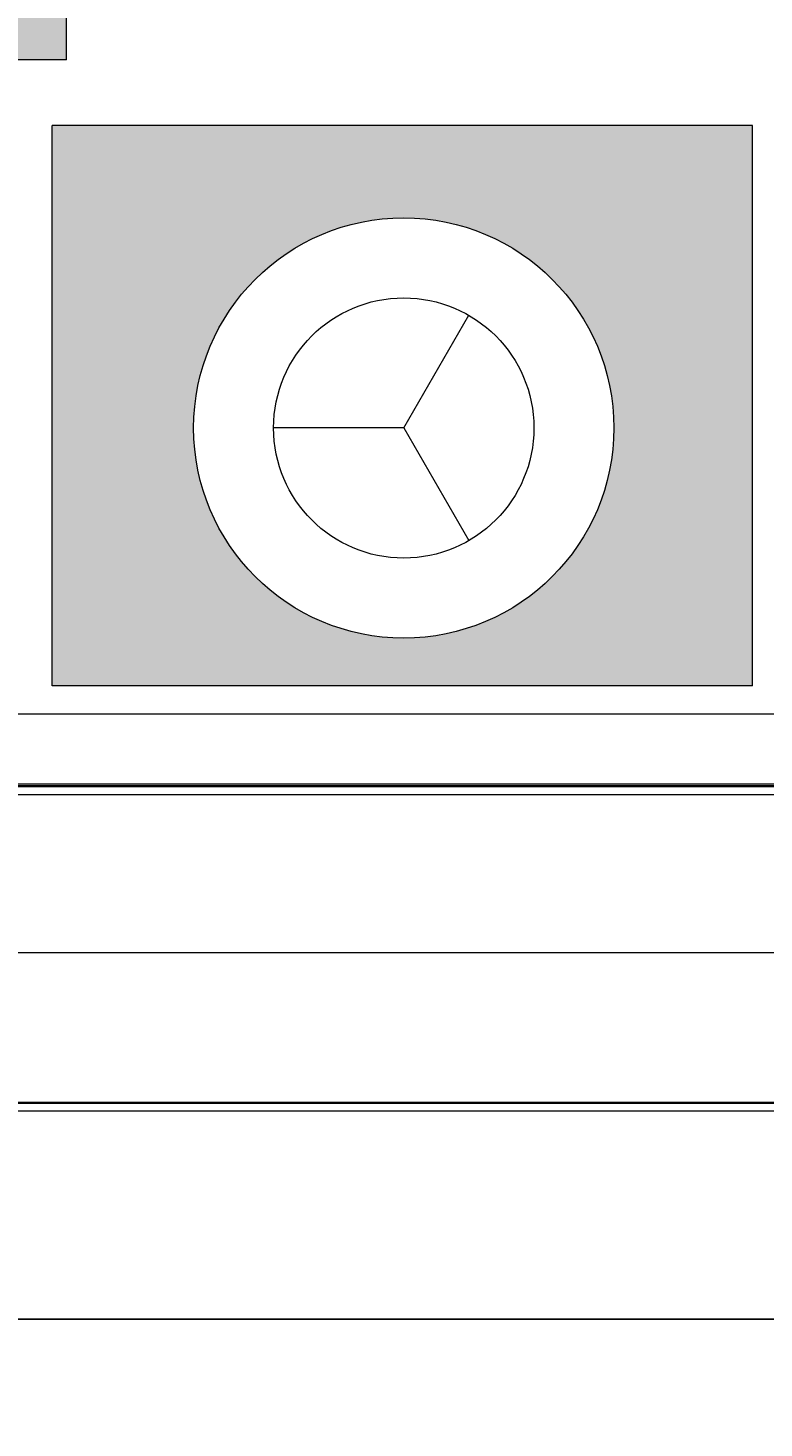
# Model space of a CAD drawing. Units: millimetres. Extents: x 27017497 to 27018854, y 7058029 to 7059154.
# Tile 25 of 91: x 27017732 to 27017753, y 7058124 to 7058163. Entities that reach past the tile are written whole.
import ezdxf

# ---------------------------------------------------------------- set-up
doc = ezdxf.new("R2010")
doc.units = ezdxf.units.MM
for name, color, linetype, lineweight in [('A-ANNO-DIMS', 2, 'Continuous', 18), ('A-FURN', 8, 'Continuous', 18), ('A-GLAZ', 4, 'Continuous', 18), ('A-WALL', 7, 'Continuous', 35)]:
    doc.layers.add(name, color=color, linetype=linetype, lineweight=lineweight)
doc.layers.add('A-FURN-PATT', color=177, linetype='Continuous', lineweight=13, true_color=0x293189)
doc.styles.get("Standard").update_dxf_attribs({"font": 'arial.ttf'})
doc.dimstyles.get("Standard").update_dxf_attribs({"dimtxt": 0.18, "dimasz": 0.18, "dimexe": 0.18, "dimexo": 0.0625, "dimgap": 0.09, "dimtad": 0, "dimtih": 1, "dimtoh": 1, "dimdec": 4, "dimzin": 0, "dimdsep": 46, "dimtxsty": 'Standard', "dimcen": 0.09, "dimadec": 0, "dimazin": 0, "dimtfac": 1, "dimtdec": 4, "dimtofl": 0, "dimtmove": 0, "dimatfit": 3, "dimfxl": 1, "dimtolj": 1, "dimtzin": 0, "dimarcsym": 0})

# ---------------------------------------------------------------- blocks, each defined once
blk = doc.blocks.new('CAMMAT')
for p, q in [((1.27313, 0), (-1.27313, 0)), ((1.27313, -0.05), (-1.27313, -0.05)), ((-1.18, -0.07), (-1.18, -0.47)), ((-1.18, -0.07), (-0.68, -0.07)), ((-0.68, -0.07), (-0.68, -0.47)), ((-0.93104, -0.2541), (-0.97748, -0.17366)), ((-0.93104, -0.2541), (-0.97748, -0.33455)), ((-0.93104, -0.2541), (-0.83815, -0.2541)), ((-1.18, -0.47), (-0.68, -0.47)), ((-0.6904, -0.51693), (-0.6904, -0.8)), ((-0.6904, -0.51693), (0.68256, -0.51693))]:
    blk.add_line(p, q)
for radius in [0.15, 0.09289]:
    blk.add_circle((-0.93104, -0.2541), radius)
blk = doc.blocks.new('WINDOW-SINGLE-LIGHT')
blk.add_lwpolyline([(36, 4.5), (36, 0), (0, 0), (0, 9), (36, 9), (36, 4.5), (0, 4.5)])
blk = doc.blocks.new('*D25')
at = {"layer": 'A-ANNO-DIMS', "color": 0, "lineweight": -2, "transparency": 16777216}
for p, q in [((27017654.932, 7058141.917), (27017654.932, 7058126.587)), ((27017756.349, 7058141.917), (27017756.349, 7058126.587)), ((27017655.112, 7058126.767), (27017704.753, 7058126.767)), ((27017756.169, 7058126.767), (27017706.528, 7058126.767))]:
    blk.add_line(p, q, dxfattribs=at)
at = {"layer": 'A-ANNO-DIMS', "color": 0, "transparency": 16777216}
for points in [[(27017655.112, 7058126.797), (27017655.112, 7058126.737), (27017654.932, 7058126.767)], [(27017756.169, 7058126.797), (27017756.169, 7058126.737), (27017756.349, 7058126.767)]]:
    blk.add_solid(points, dxfattribs=at)
at = {"layer": 'Defpoints', "color": 0, "transparency": 16777216}
for p in [(27017654.932, 7058141.98), (27017756.349, 7058141.98), (27017654.932, 7058126.767)]:
    blk.add_point(p, dxfattribs=at)
at = {"layer": 'A-ANNO-DIMS', "color": 0, "transparency": 16777216, "insert": (27017705.64, 7058126.767), "char_height": 0.18, "attachment_point": 5}
blk.add_mtext('\\A1;BED 101 TYP.', dxfattribs=at)
blk = doc.blocks.new('*D47')
at = {"layer": 'A-ANNO-DIMS', "color": 0, "lineweight": -2, "transparency": 16777216}
for p, q in [((27017561.166, 7058294.35), (27017561.166, 7058028.6)), ((27018790.606, 7058294.35), (27018790.606, 7058028.6)), ((27017561.346, 7058028.78), (27018175.431, 7058028.78)), ((27018790.426, 7058028.78), (27018176.341, 7058028.78))]:
    blk.add_line(p, q, dxfattribs=at)
at = {"layer": 'A-ANNO-DIMS', "color": 0, "transparency": 16777216}
for points in [[(27017561.346, 7058028.81), (27017561.346, 7058028.75), (27017561.166, 7058028.78)], [(27018790.426, 7058028.81), (27018790.426, 7058028.75), (27018790.606, 7058028.78)]]:
    blk.add_solid(points, dxfattribs=at)
at = {"layer": 'Defpoints', "color": 0, "transparency": 16777216}
for p in [(27017561.166, 7058294.412), (27018790.606, 7058294.412), (27018790.606, 7058028.78)]:
    blk.add_point(p, dxfattribs=at)
at = {"layer": 'A-ANNO-DIMS', "color": 0, "transparency": 16777216, "insert": (27018175.886, 7058028.78), "char_height": 0.18, "attachment_point": 5}
blk.add_mtext('\\A1;1229.4', dxfattribs=at)
blk = doc.blocks.new('*D48')
at = {"layer": 'A-ANNO-DIMS', "color": 0, "lineweight": -2, "transparency": 16777216}
for p, q in [((27018463.498, 7058622.912), (27017497.536, 7058622.912)), ((27017497.716, 7058622.732), (27017497.716, 7058357.753)), ((27017497.716, 7058092.41), (27017497.716, 7058357.389)), ((27018555.129, 7058092.23), (27017497.536, 7058092.23))]:
    blk.add_line(p, q, dxfattribs=at)
at = {"layer": 'A-ANNO-DIMS', "color": 0, "transparency": 16777216}
for points in [[(27017497.686, 7058622.732), (27017497.746, 7058622.732), (27017497.716, 7058622.912)], [(27017497.686, 7058092.41), (27017497.746, 7058092.41), (27017497.716, 7058092.23)]]:
    blk.add_solid(points, dxfattribs=at)
at = {"layer": 'Defpoints', "color": 0, "transparency": 16777216}
for p in [(27018463.561, 7058622.912), (27017497.716, 7058092.23), (27018555.192, 7058092.23)]:
    blk.add_point(p, dxfattribs=at)
at = {"layer": 'A-ANNO-DIMS', "color": 0, "transparency": 16777216, "insert": (27017497.716, 7058357.571), "char_height": 0.18, "attachment_point": 5}
blk.add_mtext('\\A1;530.7', dxfattribs=at)

msp = doc.modelspace()

# ---------------------------------------------------------------- hatches: boundary and pattern name
at = {"layer": 'A-FURN-PATT'}
h = msp.add_hatch(color=256, dxfattribs=at)
h.dxf.hatch_style = 1
h.paths.add_polyline_path([(27017731.53, 7058218.852, 0.414214), (27017729.937, 7058220.445), (27017681.344, 7058220.445, 0.414214), (27017679.751, 7058218.852), (27017679.751, 7058174.658), (27017683.647, 7058174.959), (27017687.23, 7058175.46), (27017689.748, 7058176.196), (27017691.461, 7058177.277), (27017692.628, 7058178.816), (27017693.508, 7058180.922), (27017694.36, 7058183.707), (27017694.963, 7058180.902), (27017695.506, 7058178.662), (27017696.096, 7058176.759), (27017696.84, 7058174.966), (27017697.847, 7058173.059), (27017699.222, 7058170.809), (27017701.073, 7058167.99), (27017703.508, 7058164.376), (27017705.943, 7058167.99), (27017707.794, 7058170.809), (27017709.169, 7058173.059), (27017710.176, 7058174.966), (27017710.92, 7058176.759), (27017711.51, 7058178.662), (27017712.053, 7058180.902), (27017712.656, 7058183.707), (27017713.508, 7058180.922), (27017714.388, 7058178.816), (27017715.555, 7058177.277), (27017717.268, 7058176.196), (27017719.786, 7058175.46), (27017723.369, 7058174.959), (27017728.274, 7058174.58), (27017731.53, 7058174.396)])
h.paths.add_polyline_path([(27017723.369, 7058174.959), (27017719.786, 7058175.46), (27017717.268, 7058176.196), (27017715.555, 7058177.277), (27017714.388, 7058178.816), (27017713.508, 7058180.922), (27017712.656, 7058183.707), (27017712.053, 7058180.902), (27017711.51, 7058178.662), (27017710.92, 7058176.759), (27017710.176, 7058174.966), (27017709.169, 7058173.059), (27017707.794, 7058170.809), (27017705.943, 7058167.99), (27017703.508, 7058164.376), (27017734.763, 7058174.214), (27017728.274, 7058174.58)])
h.paths.add_polyline_path([(27017696.84, 7058174.966), (27017696.096, 7058176.759), (27017695.506, 7058178.662), (27017694.963, 7058180.902), (27017694.36, 7058183.707), (27017693.508, 7058180.922), (27017692.628, 7058178.816), (27017691.461, 7058177.277), (27017689.748, 7058176.196), (27017687.23, 7058175.46), (27017683.647, 7058174.959), (27017679.751, 7058174.658), (27017678.741, 7058174.58), (27017672.253, 7058174.214), (27017703.508, 7058164.376), (27017701.073, 7058167.99), (27017699.222, 7058170.809), (27017697.847, 7058173.059)])
h.paths.add_polyline_path([(27017678.454, 7058172.262), (27017678.454, 7058162.569), (27017733.139, 7058162.569), (27017733.139, 7058173.703), (27017703.508, 7058164.376)])
h.paths.add_polyline_path([(27017730.145, 7058158.291, 0.41419), (27017728.95, 7058159.485), (27017707.491, 7058159.485, 0.414214), (27017706.296, 7058158.29), (27017706.296, 7058148.731, 0.414214), (27017707.491, 7058147.536), (27017728.95, 7058147.536, 0.414237), (27017730.145, 7058148.731)], flags=0)
h.paths.add_polyline_path([(27017731.53, 7058162.569), (27017679.751, 7058162.569), (27017679.751, 7058146.361, 0.414214), (27017681.344, 7058144.768), (27017729.937, 7058144.768, 0.414214), (27017731.53, 7058146.361)])
h.paths.add_polyline_path([(27017703.354, 7058159.485, -0.41419), (27017704.549, 7058158.291), (27017704.549, 7058148.731, -0.414237), (27017703.354, 7058147.536), (27017681.894, 7058147.536, -0.41419), (27017680.699, 7058148.731), (27017680.699, 7058158.29, -0.414237), (27017681.894, 7058159.485)], flags=0)
h.paths.add_polyline_path([(27017707.491, 7058159.485), (27017728.95, 7058159.485, -0.41419), (27017730.145, 7058158.291), (27017730.145, 7058148.731, -0.414237), (27017728.95, 7058147.536), (27017707.491, 7058147.536, -0.414214), (27017706.296, 7058148.731), (27017706.296, 7058158.29, -0.414214)], flags=16)
h.paths.add_polyline_path([(27017704.549, 7058158.291, 0.41419), (27017703.354, 7058159.485), (27017681.894, 7058159.485, 0.414237), (27017680.699, 7058158.29), (27017680.699, 7058148.731, 0.41419), (27017681.894, 7058147.536), (27017703.354, 7058147.536, 0.414237), (27017704.549, 7058148.731)], flags=16)
h.paths.add_polyline_path([(27017752.64, 7058160.7), (27017732.725, 7058160.7), (27017732.725, 7058144.768), (27017752.64, 7058144.768)])
h.paths.add_polyline_path([(27017748.698, 7058152.101, -1), (27017736.749, 7058152.101, -1)], flags=16)
h.paths.add_polyline_path([(27017746.424, 7058152.101, -1), (27017739.024, 7058152.101, -1)], flags=0)
h.paths.add_polyline_path([(27017678.556, 7058160.7), (27017658.641, 7058160.7), (27017658.641, 7058144.768), (27017678.556, 7058144.768)])
h.paths.add_polyline_path([(27017674.806, 7058152.101, -1), (27017662.857, 7058152.101, -1)], flags=16)
h.paths.add_polyline_path([(27017672.531, 7058152.101, -1), (27017665.131, 7058152.101, -1)], flags=0)

# ---------------------------------------------------------------- linework, layer by layer
at = {"layer": 'A-WALL'}
for p, q in [((27017622.666, 7058141.912), (27017802.166, 7058141.912)), ((27017613.666, 7058132.912), (27017802.166, 7058132.912)), ((27017613.666, 7058132.912), (27017802.166, 7058132.912))]:
    msp.add_line(p, q, dxfattribs=at)

# ---------------------------------------------------------------- block references
at = {"layer": 'A-FURN', "xscale": 39.82996475819422, "yscale": 39.82996475819422, "zscale": 39.82996475819422, "rotation": 180}
msp.add_blockref('CAMMAT', (27017705.64, 7058141.98), dxfattribs=at)
at = {"layer": 'A-GLAZ'}
msp.add_blockref('WINDOW-SINGLE-LIGHT', (27017727.724, 7058132.679), dxfattribs=at)

# ---------------------------------------------------------------- dimensions: what is measured, and where the dimension line sits
at = {"layer": 'A-ANNO-DIMS'}
dim = msp.add_linear_dim(base=(27017497.716, 7058092.23), p1=(27018463.561, 7058622.912), p2=(27018555.192, 7058092.23), angle=90, dimstyle='Standard', override={"dimdec": 1, "dimlfac": 1, "dimrnd": 0, "dimzin": 0, "dimdsep": 46, "dimlunit": 2}, dxfattribs=at)
dim.commit()
dim.dimension.update_dxf_attribs({"geometry": '*D48', "text_midpoint": (27017497.716, 7058357.571)})
dim = msp.add_linear_dim(base=(27018790.606, 7058028.78), p1=(27017561.166, 7058294.412), p2=(27018790.606, 7058294.412), dimstyle='Standard', override={"dimdec": 1, "dimlfac": 1, "dimrnd": 0, "dimzin": 0, "dimdsep": 46, "dimlunit": 2}, dxfattribs=at)
dim.commit()
dim.dimension.update_dxf_attribs({"geometry": '*D47', "text_midpoint": (27018175.886, 7058028.78)})
dim = msp.add_linear_dim(base=(27017654.932, 7058126.767), p1=(27017756.349, 7058141.98), p2=(27017654.932, 7058141.98), angle=180, text='BED <> TYP.', dimstyle='Standard', override={"dimdec": 0, "dimlfac": 1, "dimrnd": 0, "dimzin": 0, "dimdsep": 46, "dimlunit": 2}, dxfattribs=at)
dim.commit()
dim.dimension.update_dxf_attribs({"geometry": '*D25', "text_midpoint": (27017705.64, 7058126.767)})

doc.saveas('drawing.dxf')
